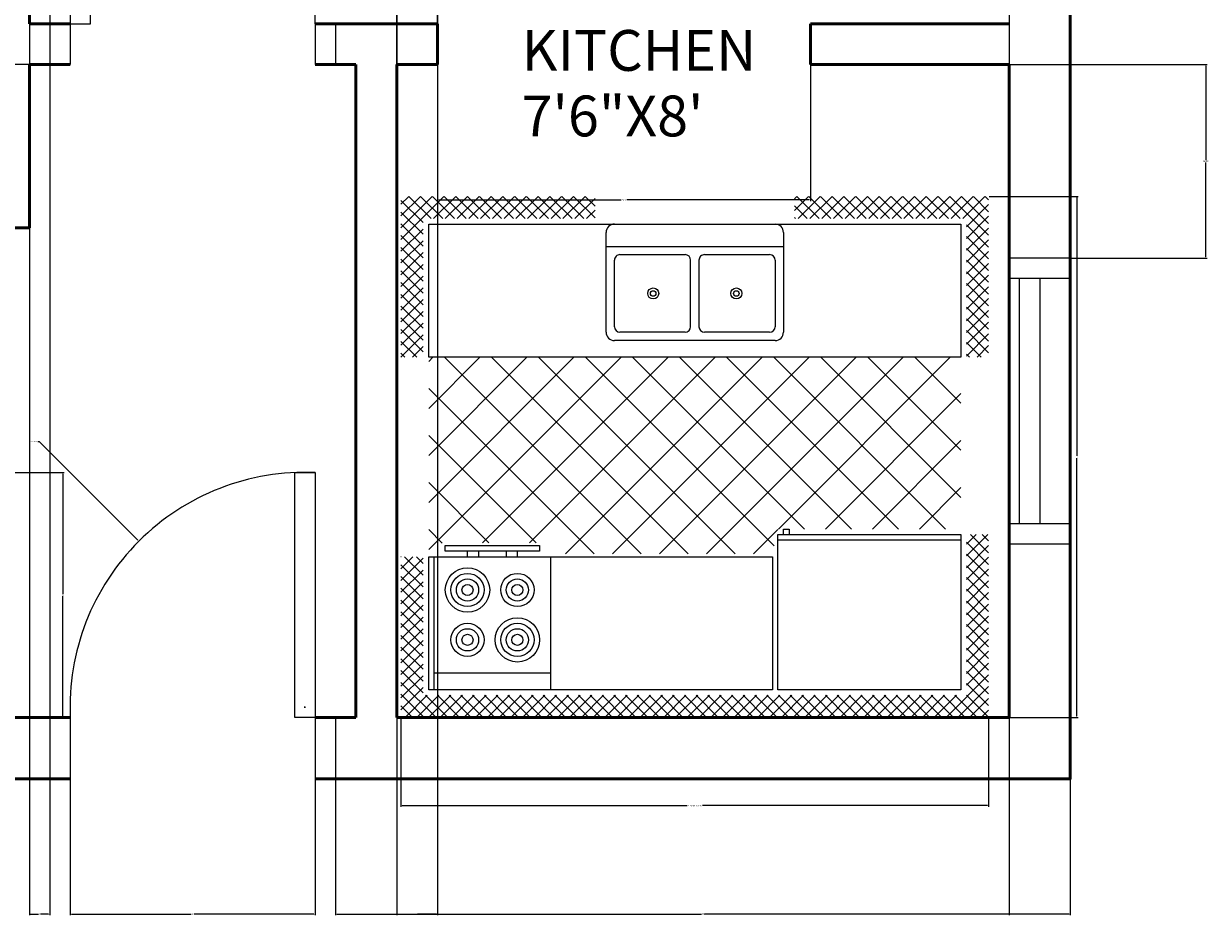
# Model space of a CAD drawing. Units: inches. Extents: x 2630 to 2982, y 643 to 1079.
# Tile 2 of 4: x 2808 to 2982, y 643 to 774. Entities that reach past the tile are written whole.
import ezdxf

# ---------------------------------------------------------------- set-up
doc = ezdxf.new("R2010")
doc.units = ezdxf.units.IN
for name, color, linetype, lineweight in [('A-ANNO-DIMS', 2, 'Continuous', 18), ('A-AREA-IDEN', 7, 'Continuous', 25), ('A-DOOR', 3, 'Continuous', 25), ('A-FLOR-FIXT', 9, 'Continuous', 18), ('A-GLAZ', 4, 'Continuous', 18), ('A-WALL', 7, 'Continuous', 50)]:
    doc.layers.add(name, color=color, linetype=linetype, lineweight=lineweight)
doc.styles.get("Standard").update_dxf_attribs({"font": 'arial.ttf'})
doc.dimstyles.get("Standard").update_dxf_attribs({"dimtxt": 0.18, "dimasz": 0.18, "dimexe": 0.18, "dimexo": 0.0625, "dimgap": 0.09, "dimtad": 0, "dimtih": 1, "dimtoh": 1, "dimdec": 4, "dimzin": 0, "dimdsep": 46, "dimtxsty": 'Standard', "dimcen": 0.09, "dimadec": 0, "dimazin": 0, "dimtfac": 1, "dimtdec": 4, "dimtofl": 0, "dimtmove": 0, "dimatfit": 3, "dimfxl": 1, "dimtolj": 1, "dimtzin": 0, "dimarcsym": 0})

# ---------------------------------------------------------------- blocks, each defined once
blk = doc.blocks.new('Kitchen Layout - 7 x 8 ft')
for p, q in [((-5, 81.32), (2.68, 89)), ((-5, 83.44), (0.56, 89)), ((-5, 85.56), (-1.56, 89)), ((-5, 87.68), (-3.68, 89)), ((-1, 84.97), (-5, 88.97)), ((1.09, 85), (-2.91, 89)), ((3.21, 85), (-0.79, 89)), ((0.81, 85), (4.81, 89)), ((5.34, 85), (1.34, 89)), ((2.93, 85), (6.93, 89)), ((7.46, 85), (3.46, 89)), ((5.05, 85), (9.05, 89)), ((9.58, 85), (5.58, 89)), ((7.17, 85), (11.17, 89)), ((11.7, 85), (7.7, 89)), ((9.29, 85), (13.29, 89)), ((13.82, 85), (9.82, 89)), ((11.41, 85), (15.41, 89)), ((15.94, 85), (11.94, 89)), ((13.53, 85), (17.53, 89)), ((18.06, 85), (14.06, 89)), ((15.65, 85), (19.65, 89)), ((20.18, 85), (16.18, 89)), ((17.78, 85), (21.78, 89)), ((22.31, 85), (18.31, 89)), ((19.9, 85), (23.9, 89)), ((24.43, 85), (20.43, 89)), ((22.02, 85), (26.02, 89)), ((26.55, 85), (22.55, 89)), ((24.14, 85), (28.14, 89)), ((28.67, 85), (24.67, 89)), ((26.26, 85), (30.26, 89)), ((30.79, 85), (26.79, 89)), ((28.38, 85), (32.38, 89)), ((32.91, 85), (28.91, 89)), ((30.5, 85), (34.5, 89)), ((35.03, 85), (31.03, 89)), ((32.63, 85), (36.63, 89)), ((37.16, 85), (33.16, 89)), ((34.75, 85), (38.75, 89)), ((39.28, 85), (35.28, 89)), ((36.87, 85), (40.87, 89)), ((41.4, 85), (37.4, 89)), ((38.99, 85), (42.99, 89)), ((43.52, 85), (39.52, 89)), ((41.11, 85), (45.11, 89)), ((45.64, 85), (41.64, 89)), ((43.23, 85), (47.23, 89)), ((47.76, 85), (43.76, 89)), ((45.35, 85), (49.35, 89)), ((49.88, 85), (45.88, 89)), ((47.47, 85), (51.47, 89)), ((52, 85), (48, 89)), ((49.6, 85), (53.6, 89)), ((54.13, 85), (50.13, 89)), ((51.72, 85), (55.72, 89)), ((56.25, 85), (52.25, 89)), ((53.84, 85), (57.84, 89)), ((58.37, 85), (54.37, 89)), ((55.96, 85), (59.96, 89)), ((60.49, 85), (56.49, 89)), ((58.08, 85), (62.08, 89)), ((62.61, 85), (58.61, 89)), ((60.2, 85), (64.2, 89)), ((64.73, 85), (60.73, 89)), ((62.32, 85), (66.32, 89)), ((66.85, 85), (62.85, 89)), ((64.45, 85), (68.45, 89)), ((68.97, 85), (64.97, 89)), ((66.57, 85), (70.57, 89)), ((71.1, 85), (67.1, 89)), ((68.69, 85), (72.69, 89)), ((73.22, 85), (69.22, 89)), ((70.81, 85), (74.81, 89)), ((75.34, 85), (71.34, 89)), ((72.93, 85), (76.93, 89)), ((77.46, 85), (73.46, 89)), ((75.05, 85), (79.05, 89)), ((79.58, 85), (75.58, 89)), ((77.17, 85), (81.17, 89)), ((81.7, 85), (77.7, 89)), ((79.29, 85), (83.29, 89)), ((83.82, 85), (79.82, 89)), ((81.42, 85), (85.42, 89)), ((85.95, 85), (81.95, 89)), ((83.54, 85), (87.54, 89)), ((88.07, 85), (84.07, 89)), ((85.66, 85), (89.66, 89)), ((90.19, 85), (86.19, 89)), ((87.78, 85), (91.78, 89)), ((92.31, 85), (88.31, 89)), ((89.9, 85), (93.9, 89)), ((94.43, 85), (90.43, 89)), ((92.02, 85), (96.02, 89)), ((96.55, 85), (92.55, 89)), ((94.14, 85), (98.14, 89)), ((101, 82.67), (94.67, 89)), ((96.27, 85), (100.27, 89)), ((101, 84.79), (96.79, 89)), ((97, 83.61), (101, 87.61)), ((101, 86.92), (98.92, 89)), ((-1, 82.85), (-5, 86.85)), ((97, 81.49), (101, 85.49)), ((-1, 80.73), (-5, 84.73)), ((34, 84), (96, 84)), ((34, 60), (34, 84)), ((96, 84), (96, 60)), ((101, 80.55), (97, 84.55)), ((97, 79.37), (101, 83.37)), ((-5, 79.19), (-1, 83.19)), ((-1, 78.61), (-5, 82.61)), ((101, 78.43), (97, 82.43)), ((97, 77.25), (101, 81.25)), ((-5, 77.07), (-1, 81.07)), ((-1, 76.49), (-5, 80.49)), ((74, 81), (95, 81)), ((101, 76.31), (97, 80.31)), ((97, 75.13), (101, 79.13)), ((-5, 74.95), (-1, 78.95)), ((-1, 74.36), (-5, 78.36)), ((101, 74.19), (97, 78.19)), ((97, 73.01), (101, 77.01)), ((-5, 72.83), (-1, 76.83)), ((-1, 72.24), (-5, 76.24)), ((101, 72.07), (97, 76.07)), ((97, 70.89), (101, 74.89)), ((-5, 70.71), (-1, 74.71)), ((-1, 70.12), (-5, 74.12)), ((101, 69.95), (97, 73.95)), ((97, 68.76), (101, 72.76)), ((-5, 68.59), (-1, 72.59)), ((-1, 68), (-5, 72)), ((101, 67.82), (97, 71.82)), ((97, 66.64), (101, 70.64)), ((-5, 66.47), (-1, 70.47)), ((-1, 65.88), (-5, 69.88)), ((101, 65.7), (97, 69.7)), ((97, 64.52), (101, 68.52)), ((-5, 64.35), (-1, 68.35)), ((-1, 63.76), (-5, 67.76)), ((101, 63.58), (97, 67.58)), ((97, 62.4), (101, 66.4)), ((-5, 62.22), (-1, 66.22)), ((-1, 61.64), (-5, 65.64)), ((101, 61.46), (97, 65.46)), ((97, 60.28), (101, 64.28)), ((-5, 60.1), (-1, 64.1)), ((-1, 59.52), (-5, 63.52)), ((-5, 57.98), (-1, 61.98)), ((100.34, 60), (97, 63.34)), ((98.84, 60), (101, 62.16)), ((-1, 57.39), (-5, 61.39)), ((-4.86, 56), (-1, 59.86)), ((96, 60), (34, 60)), ((80, 60), (80, 59)), ((82, 59), (82, 60)), ((87, 59), (87, 60)), ((89, 60), (89, 59)), ((98.22, 60), (97, 61.22)), ((100.96, 60), (101, 60.04)), ((-1.73, 56), (-5, 59.27)), ((-2.74, 56), (-1, 57.74)), ((10.4, 24), (45.9, 59.5)), ((18.88, 24), (54.38, 59.5)), ((27.37, 24), (62.87, 59.5)), ((33.03, 55.11), (37.41, 59.5)), ((67.71, 24), (33.68, 58.04)), ((35.85, 24), (71.35, 59.5)), ((76.2, 24), (40.7, 59.5)), ((84.68, 24), (49.18, 59.5)), ((93.17, 24), (57.67, 59.5)), ((61.31, 24), (96, 58.69)), ((96, 29.65), (66.15, 59.5)), ((-3.85, 56), (-5, 57.15)), ((0, 57), (33, 57)), ((31, 55), (31, 56)), ((32, 56), (32, 55)), ((44.34, 24), (77.84, 57.5)), ((52.82, 24), (86.32, 57.5)), ((96, 38.14), (76.64, 57.5)), ((96, 46.63), (85.13, 57.5)), ((96, 55.11), (93.57, 57.54)), ((0, 30.57), (24.43, 55)), ((0, 39.06), (15.94, 55)), ((0, 47.54), (7.46, 55)), ((1.91, 24), (32.91, 55)), ((33.77, 24), (2.77, 55)), ((42.26, 24), (11.26, 55)), ((50.74, 24), (19.74, 55)), ((59.23, 24), (28.23, 55)), ((32, 55), (31, 55)), ((25.29, 24), (0, 49.29)), ((69.79, 24), (96, 50.21)), ((16.8, 24), (0, 40.8)), ((78.28, 24), (96, 41.72)), ((8.32, 24), (0, 32.32)), ((86.76, 24), (96, 33.24)), ((-5, 21.92), (-2.92, 24)), ((-5, 19.8), (-1, 23.8)), ((-1, 21.33), (-3.67, 24)), ((-1, 23.45), (-1.55, 24)), ((0, 24), (96, 24)), ((0, 0), (0, 24)), ((95.25, 24), (96, 24.75)), ((96, 24), (96, 0)), ((97, 22.1), (98.9, 24)), ((97, 19.97), (101, 23.97)), ((101, 21.16), (98.16, 24)), ((101, 23.28), (100.28, 24)), ((-1, 19.21), (-5, 23.21)), ((-5, 17.68), (-1, 21.68)), ((101, 19.03), (97, 23.03)), ((97, 17.85), (101, 21.85)), ((-1, 17.09), (-5, 21.09)), ((-5, 15.55), (-1, 19.55)), ((101, 16.91), (97, 20.91)), ((97, 15.73), (101, 19.73)), ((-1, 14.97), (-5, 18.97)), ((-5, 13.43), (-1, 17.43)), ((47.25, 6.5), (47.25, 18.5)), ((48.75, 18.5), (48.75, 6.5)), ((101, 14.79), (97, 18.79)), ((97, 13.61), (101, 17.61)), ((-1, 12.85), (-5, 16.85)), ((-5, 11.31), (-1, 15.31)), ((101, 12.67), (97, 16.67)), ((97, 11.49), (101, 15.49)), ((-1, 10.73), (-5, 14.73)), ((-5, 9.19), (-1, 13.19)), ((101, 10.55), (97, 14.55)), ((97, 9.37), (101, 13.37)), ((-1, 8.6), (-5, 12.6)), ((-5, 7.07), (-1, 11.07)), ((101, 8.43), (97, 12.43)), ((97, 7.25), (101, 11.25)), ((-1, 6.48), (-5, 10.48)), ((-5, 4.95), (-1, 8.95)), ((101, 6.31), (97, 10.31)), ((97, 5.12), (101, 9.12)), ((-1, 4.36), (-5, 8.36)), ((-5, 2.83), (-1, 6.83)), ((101, 4.18), (97, 8.18)), ((97, 3), (101, 7)), ((-1, 2.24), (-5, 6.24)), ((-5, 0.71), (-1, 4.71)), ((101, 2.06), (97, 6.06)), ((97, 0.88), (101, 4.88)), ((-1, 0.12), (-5, 4.12)), ((-5, -1.42), (-1, 2.58)), ((64, 4), (32, 4)), ((93.24, -5), (101, 2.76)), ((101, -0.06), (97, 3.94)), ((2, -5), (-5, 2)), ((-5, -3.54), (-1, 0.46)), ((96, 0), (0, 0)), ((95.36, -5), (101, 0.64)), ((101, -2.18), (97, 1.82)), ((-0.12, -5), (-5, -0.12)), ((-4.34, -5), (-0.34, -1)), ((-2.22, -5), (1.78, -1)), ((-0.1, -5), (3.9, -1)), ((4.12, -5), (0.12, -1)), ((2.02, -5), (6.02, -1)), ((6.24, -5), (2.24, -1)), ((4.14, -5), (8.14, -1)), ((8.36, -5), (4.36, -1)), ((6.27, -5), (10.27, -1)), ((10.48, -5), (6.48, -1)), ((8.39, -5), (12.39, -1)), ((12.6, -5), (8.6, -1)), ((10.51, -5), (14.51, -1)), ((14.73, -5), (10.73, -1)), ((12.63, -5), (16.63, -1)), ((16.85, -5), (12.85, -1)), ((14.75, -5), (18.75, -1)), ((18.97, -5), (14.97, -1)), ((16.87, -5), (20.87, -1)), ((21.09, -5), (17.09, -1)), ((18.99, -5), (22.99, -1)), ((23.21, -5), (19.21, -1)), ((21.11, -5), (25.11, -1)), ((25.33, -5), (21.33, -1)), ((23.24, -5), (27.24, -1)), ((27.45, -5), (23.45, -1)), ((25.36, -5), (29.36, -1)), ((29.57, -5), (25.57, -1)), ((30, -3.3), (27.7, -1)), ((30, -1.18), (29.82, -1)), ((66, -2.54), (67.54, -1)), ((66, -4.66), (69.66, -1)), ((69.88, -5), (66, -1.12)), ((67.78, -5), (71.78, -1)), ((72, -5), (68, -1)), ((69.9, -5), (73.9, -1)), ((74.12, -5), (70.12, -1)), ((72.03, -5), (76.03, -1)), ((76.24, -5), (72.24, -1)), ((74.15, -5), (78.15, -1)), ((78.36, -5), (74.36, -1)), ((76.27, -5), (80.27, -1)), ((80.49, -5), (76.49, -1)), ((78.39, -5), (82.39, -1)), ((82.61, -5), (78.61, -1)), ((80.51, -5), (84.51, -1)), ((84.73, -5), (80.73, -1)), ((82.63, -5), (86.63, -1)), ((86.85, -5), (82.85, -1)), ((84.75, -5), (88.75, -1)), ((88.97, -5), (84.97, -1)), ((86.88, -5), (90.88, -1)), ((91.09, -5), (87.09, -1)), ((89, -5), (93, -1)), ((93.21, -5), (89.21, -1)), ((91.12, -5), (95.12, -1)), ((95.34, -5), (91.34, -1)), ((97.46, -5), (93.46, -1)), ((99.58, -5), (95.58, -1)), ((101, -4.3), (97, -0.3)), ((97.48, -5), (101, -1.48)), ((-2.25, -5), (-5, -2.25)), ((27.48, -5), (30, -2.48)), ((67.76, -5), (66, -3.24)), ((99.6, -5), (101, -3.6)), ((-4.37, -5), (-5, -4.37)), ((29.6, -5), (30, -4.6))]:
    blk.add_line(p, q)
for points in [[(0, 56), (0, 84), (33, 84), (33, 56)], [(74, 60), (74, 84), (95, 84), (95, 60)], [(76, 58), (76, 59), (93, 59), (93, 58)]]:
    blk.add_lwpolyline(points, close=True)
for points in [[(32, 1.5), (32, 19.5)], [(33.5, 21), (62.5, 21)], [(34.5, 19.5), (46.25, 19.5)], [(49.75, 19.5), (61.5, 19.5)], [(64, 19.5), (64, 1.5)], [(33.5, 6.5), (33.5, 18.5)], [(62.5, 18.5), (62.5, 6.5)], [(46.25, 5.5), (34.5, 5.5)], [(61.5, 5.5), (49.75, 5.5)], [(62.5, 0), (33.5, 0)]]:
    blk.add_lwpolyline(points)
for centre, radius in [((80, 75), 4), ((80, 75), 3), ((80, 75), 2), ((89, 75), 3), ((89, 75), 2), ((80, 75), 1), ((89, 75), 1), ((80, 66), 3), ((89, 66), 4), ((89, 66), 3), ((80, 66), 2), ((80, 66), 1), ((89, 66), 2), ((89, 66), 1), ((40.5, 12.5), 1), ((40.5, 12.5), 0.5), ((55.5, 12.5), 1), ((55.5, 12.5), 0.5)]:
    blk.add_circle(centre, radius)
for centre, radius, start, end in [((33.5, 19.5), 1.5, 90, 180), ((34.5, 18.5), 1, 90, 180), ((46.25, 18.5), 1, 0, 90), ((49.75, 18.5), 1, 90, 180), ((61.5, 18.5), 1, 0, 90), ((62.5, 19.5), 1.5, 0, 90), ((34.5, 6.5), 1, 180, 270), ((46.25, 6.5), 1, 270, 0), ((49.75, 6.5), 1, 180, 270), ((61.5, 6.5), 1, 270, 0), ((33.5, 1.5), 1.5, 180, 270), ((62.5, 1.5), 1.5, 270, 0)]:
    blk.add_arc(centre, radius, start, end)
blk = doc.blocks.new('DOOR-36IN-INT')
for p, q in [((0, 6), (0, 0)), ((3, 6), (3, 0)), ((39, 6), (39, 0)), ((42, 6), (42, 0))]:
    blk.add_line(p, q)
blk.add_lwpolyline([(3, 6), (6, 6), (6, 42), (3, 42)], close=True)
blk.add_arc((4.5, 7.5), 34.53, 357.5104, 92.4896)
blk = doc.blocks.new('WIN-36IN')
for p, q in [((9, 42), (0, 42)), ((9, 39), (0, 39)), ((4.5, 3), (4.5, 39)), ((7.5, 3), (7.5, 39)), ((0, 3), (9, 3)), ((0, 0), (9, 0))]:
    blk.add_line(p, q)
blk = doc.blocks.new('*D19')
at = {"layer": 'A-ANNO-DIMS', "color": 0, "lineweight": -2, "transparency": 16777216}
for p, q in [((2811.7, 810.29), (2805.22, 810.29)), ((2805.4, 810.11), (2805.4, 789.26)), ((2805.4, 768.05), (2805.4, 788.89)), ((2811.7, 767.87), (2805.22, 767.87))]:
    blk.add_line(p, q, dxfattribs=at)
at = {"layer": 'A-ANNO-DIMS', "color": 0, "transparency": 16777216}
for points in [[(2805.37, 810.11), (2805.43, 810.11), (2805.4, 810.29)], [(2805.37, 768.05), (2805.43, 768.05), (2805.4, 767.87)]]:
    blk.add_solid(points, dxfattribs=at)
at = {"layer": 'Defpoints', "color": 0, "transparency": 16777216}
for p in [(2805.4, 810.29), (2811.77, 810.29), (2811.77, 767.87)]:
    blk.add_point(p, dxfattribs=at)
at = {"layer": 'A-ANNO-DIMS', "color": 0, "transparency": 16777216, "insert": (2805.4, 789.08), "char_height": 0.18, "attachment_point": 5}
blk.add_mtext('\\A1;DOOR D1 42 TYP.', dxfattribs=at)
blk = doc.blocks.new('*D35')
at = {"layer": 'A-ANNO-DIMS', "color": 0, "lineweight": -2, "transparency": 16777216}
for p, q in [((2863.38, 671.8), (2863.38, 658.73)), ((2949.76, 671.8), (2949.76, 658.73)), ((2863.56, 658.91), (2905.44, 658.91)), ((2949.58, 658.91), (2907.7, 658.91))]:
    blk.add_line(p, q, dxfattribs=at)
at = {"layer": 'A-ANNO-DIMS', "color": 0, "transparency": 16777216}
for points in [[(2863.56, 658.94), (2863.56, 658.88), (2863.38, 658.91)], [(2949.58, 658.94), (2949.58, 658.88), (2949.76, 658.91)]]:
    blk.add_solid(points, dxfattribs=at)
at = {"layer": 'Defpoints', "color": 0, "transparency": 16777216}
for p in [(2863.38, 671.87), (2949.76, 671.87), (2863.38, 658.91)]:
    blk.add_point(p, dxfattribs=at)
at = {"layer": 'A-ANNO-DIMS', "color": 0, "transparency": 16777216, "insert": (2906.57, 658.91), "char_height": 0.18, "attachment_point": 5}
blk.add_mtext('\\A1;KITCHEN UNIT 86', dxfattribs=at)
blk = doc.blocks.new('*D36')
at = {"layer": 'A-ANNO-DIMS', "color": 0, "lineweight": -2, "transparency": 16777216}
for p, q in [((2949.82, 748.47), (2962.9, 748.47)), ((2962.72, 748.29), (2962.72, 710.35)), ((2962.72, 672.05), (2962.72, 709.99)), ((2949.82, 671.87), (2962.9, 671.87))]:
    blk.add_line(p, q, dxfattribs=at)
at = {"layer": 'A-ANNO-DIMS', "color": 0, "transparency": 16777216}
for points in [[(2962.69, 748.29), (2962.75, 748.29), (2962.72, 748.47)], [(2962.69, 672.05), (2962.75, 672.05), (2962.72, 671.87)]]:
    blk.add_solid(points, dxfattribs=at)
at = {"layer": 'Defpoints', "color": 0, "transparency": 16777216}
for p in [(2949.76, 748.47), (2949.76, 671.87), (2962.72, 671.87)]:
    blk.add_point(p, dxfattribs=at)
at = {"layer": 'A-ANNO-DIMS', "color": 0, "transparency": 16777216, "insert": (2962.72, 710.17), "char_height": 0.18, "attachment_point": 5}
blk.add_mtext('\\A1;77', dxfattribs=at)
blk = doc.blocks.new('*D48')
at = {"layer": 'A-ANNO-DIMS', "color": 0, "lineweight": -2, "transparency": 16777216}
for p, q in [((2952.83, 767.87), (2981.86, 767.87)), ((2981.68, 767.69), (2981.68, 753.81)), ((2981.68, 739.57), (2981.68, 753.45)), ((2961.83, 739.39), (2981.86, 739.39))]:
    blk.add_line(p, q, dxfattribs=at)
at = {"layer": 'A-ANNO-DIMS', "color": 0, "transparency": 16777216}
for points in [[(2981.65, 767.69), (2981.71, 767.69), (2981.68, 767.87)], [(2981.65, 739.57), (2981.71, 739.57), (2981.68, 739.39)]]:
    blk.add_solid(points, dxfattribs=at)
at = {"layer": 'Defpoints', "color": 0, "transparency": 16777216}
for p in [(2952.77, 767.87), (2981.68, 767.87), (2961.77, 739.39)]:
    blk.add_point(p, dxfattribs=at)
at = {"layer": 'A-ANNO-DIMS', "color": 0, "transparency": 16777216, "insert": (2981.68, 753.63), "char_height": 0.18, "attachment_point": 5}
blk.add_mtext('\\A1;28.475', dxfattribs=at)
blk = doc.blocks.new('*D49')
at = {"layer": 'A-ANNO-DIMS', "color": 0, "lineweight": -2, "transparency": 16777216}
for p, q in [((2853.77, 662.8), (2853.77, 642.78)), ((2961.77, 662.8), (2961.77, 642.78)), ((2853.95, 642.96), (2907.49, 642.96)), ((2961.59, 642.96), (2908.05, 642.96))]:
    blk.add_line(p, q, dxfattribs=at)
at = {"layer": 'A-ANNO-DIMS', "color": 0, "transparency": 16777216}
for points in [[(2853.95, 642.99), (2853.95, 642.93), (2853.77, 642.96)], [(2961.59, 642.99), (2961.59, 642.93), (2961.77, 642.96)]]:
    blk.add_solid(points, dxfattribs=at)
at = {"layer": 'Defpoints', "color": 0, "transparency": 16777216}
for p in [(2853.77, 662.87), (2961.77, 662.87), (2961.77, 642.96)]:
    blk.add_point(p, dxfattribs=at)
at = {"layer": 'A-ANNO-DIMS', "color": 0, "transparency": 16777216, "insert": (2907.77, 642.96), "char_height": 0.18, "attachment_point": 5}
blk.add_mtext('\\A1;108', dxfattribs=at)
blk = doc.blocks.new('*D50')
at = {"layer": 'A-ANNO-DIMS', "color": 0, "lineweight": -2, "transparency": 16777216}
for p, q in [((2814.77, 662.8), (2814.77, 642.78)), ((2850.77, 662.8), (2850.77, 642.78)), ((2814.95, 642.96), (2832.55, 642.96)), ((2850.59, 642.96), (2832.99, 642.96))]:
    blk.add_line(p, q, dxfattribs=at)
at = {"layer": 'A-ANNO-DIMS', "color": 0, "transparency": 16777216}
for points in [[(2814.95, 642.99), (2814.95, 642.93), (2814.77, 642.96)], [(2850.59, 642.99), (2850.59, 642.93), (2850.77, 642.96)]]:
    blk.add_solid(points, dxfattribs=at)
at = {"layer": 'Defpoints', "color": 0, "transparency": 16777216}
for p in [(2814.77, 662.87), (2850.77, 662.87), (2850.77, 642.96)]:
    blk.add_point(p, dxfattribs=at)
at = {"layer": 'A-ANNO-DIMS', "color": 0, "transparency": 16777216, "insert": (2832.77, 642.96), "char_height": 0.18, "attachment_point": 5}
blk.add_mtext('\\A1;36', dxfattribs=at)
blk = doc.blocks.new('*D51')
at = {"layer": 'A-ANNO-DIMS', "color": 0, "lineweight": -2, "transparency": 16777216}
for p, q in [((2862.77, 875.8), (2862.77, 642.78)), ((2952.77, 875.8), (2952.77, 642.78)), ((2862.95, 642.96), (2907.55, 642.96)), ((2952.59, 642.96), (2907.99, 642.96))]:
    blk.add_line(p, q, dxfattribs=at)
at = {"layer": 'A-ANNO-DIMS', "color": 0, "transparency": 16777216}
for points in [[(2862.95, 642.99), (2862.95, 642.93), (2862.77, 642.96)], [(2952.59, 642.99), (2952.59, 642.93), (2952.77, 642.96)]]:
    blk.add_solid(points, dxfattribs=at)
at = {"layer": 'Defpoints', "color": 0, "transparency": 16777216}
for p in [(2862.77, 875.87), (2952.77, 875.87), (2952.77, 642.96)]:
    blk.add_point(p, dxfattribs=at)
at = {"layer": 'A-ANNO-DIMS', "color": 0, "transparency": 16777216, "insert": (2907.77, 642.96), "char_height": 0.18, "attachment_point": 5}
blk.add_mtext('\\A1;90', dxfattribs=at)
blk = doc.blocks.new('*D53')
at = {"layer": 'A-ANNO-DIMS', "color": 0, "lineweight": -2, "transparency": 16777216}
for p, q in [((2793.83, 707.87), (2813.86, 707.87)), ((2813.68, 707.69), (2813.68, 690.05)), ((2813.68, 672.05), (2813.68, 689.68)), ((2793.83, 671.87), (2813.86, 671.87))]:
    blk.add_line(p, q, dxfattribs=at)
at = {"layer": 'A-ANNO-DIMS', "color": 0, "transparency": 16777216}
for points in [[(2813.65, 707.69), (2813.71, 707.69), (2813.68, 707.87)], [(2813.65, 672.05), (2813.71, 672.05), (2813.68, 671.87)]]:
    blk.add_solid(points, dxfattribs=at)
at = {"layer": 'Defpoints', "color": 0, "transparency": 16777216}
for p in [(2793.77, 707.87), (2793.77, 671.87), (2813.68, 671.87)]:
    blk.add_point(p, dxfattribs=at)
at = {"layer": 'A-ANNO-DIMS', "color": 0, "transparency": 16777216, "insert": (2813.68, 689.87), "char_height": 0.18, "attachment_point": 5}
blk.add_mtext('\\A1;36', dxfattribs=at)
blk = doc.blocks.new('*D57')
at = {"layer": 'A-ANNO-DIMS', "color": 0, "lineweight": -2, "transparency": 16777216}
for p, q in [((2868.77, 767.8), (2868.77, 747.78)), ((2923.56, 767.8), (2923.56, 747.78)), ((2868.95, 747.96), (2895.77, 747.96)), ((2923.38, 747.96), (2896.56, 747.96))]:
    blk.add_line(p, q, dxfattribs=at)
at = {"layer": 'A-ANNO-DIMS', "color": 0, "transparency": 16777216}
for points in [[(2868.95, 747.99), (2868.95, 747.93), (2868.77, 747.96)], [(2923.38, 747.99), (2923.38, 747.93), (2923.56, 747.96)]]:
    blk.add_solid(points, dxfattribs=at)
at = {"layer": 'Defpoints', "color": 0, "transparency": 16777216}
for p in [(2868.77, 767.87), (2923.56, 767.87), (2868.77, 747.96)]:
    blk.add_point(p, dxfattribs=at)
at = {"layer": 'A-ANNO-DIMS', "color": 0, "transparency": 16777216, "insert": (2896.16, 747.96), "char_height": 0.18, "attachment_point": 5}
blk.add_mtext('\\A1;54.79', dxfattribs=at)
blk = doc.blocks.new('*D58')
at = {"layer": 'A-ANNO-DIMS', "color": 0, "lineweight": -2, "transparency": 16777216}
for p, q in [((2862.77, 767.93), (2862.77, 1078.96)), ((2862.95, 1078.78), (2865.62, 1078.78)), ((2868.59, 1078.78), (2865.92, 1078.78)), ((2868.77, 767.93), (2868.77, 1078.96))]:
    blk.add_line(p, q, dxfattribs=at)
at = {"layer": 'A-ANNO-DIMS', "color": 0, "transparency": 16777216}
for points in [[(2862.95, 1078.81), (2862.95, 1078.75), (2862.77, 1078.78)], [(2868.59, 1078.81), (2868.59, 1078.75), (2868.77, 1078.78)]]:
    blk.add_solid(points, dxfattribs=at)
at = {"layer": 'Defpoints', "color": 0, "transparency": 16777216}
for p in [(2868.77, 1078.78), (2862.77, 767.87), (2868.77, 767.87)]:
    blk.add_point(p, dxfattribs=at)
at = {"layer": 'A-ANNO-DIMS', "color": 0, "transparency": 16777216, "insert": (2865.77, 1078.78), "char_height": 0.18, "attachment_point": 5}
blk.add_mtext('\\A1;6', dxfattribs=at)
blk = doc.blocks.new('*D59')
at = {"layer": 'A-ANNO-DIMS', "color": 0, "lineweight": -2, "transparency": 16777216}
for p, q in [((2808.77, 929.8), (2808.77, 642.78)), ((2811.77, 929.8), (2811.77, 642.78)), ((2808.95, 642.96), (2810.12, 642.96)), ((2811.59, 642.96), (2810.42, 642.96))]:
    blk.add_line(p, q, dxfattribs=at)
at = {"layer": 'A-ANNO-DIMS', "color": 0, "transparency": 16777216}
for points in [[(2808.95, 642.99), (2808.95, 642.93), (2808.77, 642.96)], [(2811.59, 642.99), (2811.59, 642.93), (2811.77, 642.96)]]:
    blk.add_solid(points, dxfattribs=at)
at = {"layer": 'Defpoints', "color": 0, "transparency": 16777216}
for p in [(2808.77, 929.87), (2811.77, 929.87), (2811.77, 642.96)]:
    blk.add_point(p, dxfattribs=at)
at = {"layer": 'A-ANNO-DIMS', "color": 0, "transparency": 16777216, "insert": (2810.27, 642.96), "char_height": 0.18, "attachment_point": 5}
blk.add_mtext('\\A1;3', dxfattribs=at)
blk = doc.blocks.new('*D60')
at = {"layer": 'A-ANNO-DIMS', "color": 0, "lineweight": -2, "transparency": 16777216}
for p, q in [((2862.77, 923.8), (2862.77, 642.78)), ((2868.77, 923.8), (2868.77, 642.78)), ((2862.95, 642.96), (2865.62, 642.96)), ((2868.59, 642.96), (2865.92, 642.96))]:
    blk.add_line(p, q, dxfattribs=at)
at = {"layer": 'A-ANNO-DIMS', "color": 0, "transparency": 16777216}
for points in [[(2862.95, 642.99), (2862.95, 642.93), (2862.77, 642.96)], [(2868.59, 642.99), (2868.59, 642.93), (2868.77, 642.96)]]:
    blk.add_solid(points, dxfattribs=at)
at = {"layer": 'Defpoints', "color": 0, "transparency": 16777216}
for p in [(2862.77, 923.87), (2868.77, 923.87), (2868.77, 642.96)]:
    blk.add_point(p, dxfattribs=at)
at = {"layer": 'A-ANNO-DIMS', "color": 0, "transparency": 16777216, "insert": (2865.77, 642.96), "char_height": 0.18, "attachment_point": 5}
blk.add_mtext('\\A1;6', dxfattribs=at)
blk = doc.blocks.new('*D69')
at = {"layer": 'A-ANNO-DIMS', "color": 0, "lineweight": -2, "transparency": 16777216}
for p, q in [((2810.02, 712.44), (2810.2, 712.44)), ((2810.2, 712.44), (2824.72, 697.91)), ((2849.18, 673.37), (2849.36, 673.37)), ((2849.27, 673.28), (2849.27, 673.46))]:
    blk.add_line(p, q, dxfattribs=at)
at = {"layer": 'A-ANNO-DIMS', "color": 0, "transparency": 16777216}
blk.add_solid([(2824.74, 697.93), (2824.7, 697.89), (2824.85, 697.78)], dxfattribs=at)
at = {"layer": 'Defpoints', "color": 0, "transparency": 16777216}
for p in [(2824.85, 697.78), (2849.27, 673.37)]:
    blk.add_point(p, dxfattribs=at)
at = {"layer": 'A-ANNO-DIMS', "color": 0, "transparency": 16777216, "insert": (2809.34, 712.44), "char_height": 0.18, "attachment_point": 5}
blk.add_mtext('\\A1;4X R34.53', dxfattribs=at)

msp = doc.modelspace()

# ---------------------------------------------------------------- linework, layer by layer
at = {"layer": 'A-DOOR'}
for p, q in [((2811.7671, 671.8666), (2811.7671, 662.8666)), ((2814.7671, 671.8666), (2814.7671, 662.8666)), ((2850.7671, 671.8666), (2850.7671, 662.8666)), ((2853.7671, 671.8666), (2853.7671, 662.8666))]:
    msp.add_line(p, q, dxfattribs=at)
msp.add_lwpolyline([(2850.7671, 671.8666), (2847.7671, 671.8666), (2847.7671, 707.8666), (2850.7671, 707.8666)], close=True, dxfattribs=at)
msp.add_arc((2849.2671, 673.3666), 34.5326, 87.510447, 182.489553, dxfattribs=at)
at = {"layer": 'A-WALL'}
for p, q in [((2808.7671, 875.8666), (2808.7671, 773.8666)), ((2808.7671, 773.8666), (2814.7671, 773.8666)), ((2850.7671, 773.8666), (2868.7671, 773.8666)), ((2868.7671, 767.8666), (2868.7671, 773.8666)), ((2923.557, 773.8666), (2952.7671, 773.8666)), ((2923.557, 773.8666), (2923.557, 767.8666)), ((2808.7671, 767.8666), (2814.7671, 767.8666)), ((2808.7671, 767.8666), (2808.7671, 743.8666)), ((2850.7671, 767.8666), (2856.7671, 767.8666)), ((2856.7671, 671.8666), (2856.7671, 767.8666)), ((2862.7671, 671.8666), (2862.7671, 767.8666)), ((2862.7671, 767.8666), (2868.7671, 767.8666)), ((2923.557, 767.8666), (2952.7671, 767.8666)), ((2952.7671, 671.8666), (2952.7671, 767.8666)), ((2808.7671, 743.8666), (2658.7671, 743.8666)), ((2658.7671, 671.8666), (2814.7671, 671.8666)), ((2850.7671, 671.8666), (2856.7671, 671.8666)), ((2862.7671, 671.8666), (2952.7671, 671.8666))]:
    msp.add_line(p, q, dxfattribs=at)
msp.add_lwpolyline([(2850.7671, 662.8666), (2961.7671, 662.8666), (2961.7671, 1058.8666), (2649.7671, 1058.8666), (2649.7671, 662.8666), (2814.7671, 662.8666)], dxfattribs=at)

# ---------------------------------------------------------------- block references
at = {"layer": 'A-DOOR'}
msp.add_blockref('DOOR-36IN-INT', (2811.767, 767.867), dxfattribs=at)
at = {"layer": 'A-FLOR-FIXT', "xscale": 0.8148768357365197, "yscale": 0.8148768357365197, "zscale": 0.8148768357365197, "rotation": 180}
msp.add_blockref('Kitchen Layout - 7 x 8 ft', (2945.6847, 744.3907), dxfattribs=at)
at = {"layer": 'A-GLAZ', "rotation": 180}
msp.add_blockref('WIN-36IN', (2961.7672, 739.3914), dxfattribs=at)

# ---------------------------------------------------------------- texts
at = {"layer": 'A-AREA-IDEN'}
for s, p in [('KITCHEN', (2881.1094, 766.9372)), ('7\'6"X8\'', (2881.1094, 757.2987))]:
    msp.add_text(s, height=6, dxfattribs=at).set_placement(p)

# ---------------------------------------------------------------- dimensions: what is measured, and where the dimension line sits
at = {"layer": 'A-ANNO-DIMS'}
for base, p1, p2, picture, middle in [((2868.7671, 1078.7766), (2862.7671, 767.8666), (2868.7671, 767.8666), '*D58', (2865.7671, 1078.7766)), ((2811.7671, 642.9566), (2808.7671, 929.8666), (2811.7671, 929.8666), '*D59', (2810.2671, 642.9566)), ((2868.7671, 642.9566), (2862.7671, 923.8666), (2868.7671, 923.8666), '*D60', (2865.7671, 642.9566)), ((2952.7671, 642.9566), (2862.7671, 875.8666), (2952.7671, 875.8666), '*D51', (2907.7671, 642.9566)), ((2850.7671, 642.9566), (2814.7671, 662.8666), (2850.7671, 662.8666), '*D50', (2832.7671, 642.9566)), ((2961.7671, 642.9566), (2853.7671, 662.8666), (2961.7671, 662.8666), '*D49', (2907.7671, 642.9566))]:
    dim = msp.add_linear_dim(base=base, p1=p1, p2=p2, dimstyle='Standard', override={"dimdec": 0, "dimlfac": 1, "dimrnd": 0, "dimzin": 0, "dimdsep": 46, "dimlunit": 2}, dxfattribs=at)
    dim.commit()
    dim.dimension.update_dxf_attribs({"geometry": picture, "text_midpoint": middle})
for base, p1, p2, angle, text, picture, middle in [((2805.404, 810.2871), (2811.7671, 767.8666), (2811.7671, 810.2871), 90, 'DOOR D1 <> TYP.', '*D19', (2805.404, 789.0769)), ((2863.3821, 658.9101), (2949.7591, 671.8666), (2863.3821, 671.8666), 180, 'KITCHEN UNIT <>', '*D35', (2906.5706, 658.9101))]:
    dim = msp.add_linear_dim(base=base, p1=p1, p2=p2, angle=angle, text=text, dimstyle='Standard', override={"dimdec": 0, "dimlfac": 1, "dimrnd": 0, "dimzin": 0, "dimdsep": 46, "dimlunit": 2}, dxfattribs=at)
    dim.commit()
    dim.dimension.update_dxf_attribs({"geometry": picture, "text_midpoint": middle})
for base, p1, p2, angle, override, picture, middle in [((2868.7671, 747.9566), (2923.557, 767.8666), (2868.7671, 767.8666), 180, {"dimdec": 2, "dimlfac": 1, "dimrnd": 0, "dimzin": 0, "dimdsep": 46, "dimlunit": 2}, '*D57', (2896.162, 747.9566)), ((2981.6771, 767.8666), (2961.7671, 739.3915), (2952.7671, 767.8666), 90, {"dimdec": 3, "dimlfac": 1, "dimrnd": 0, "dimzin": 0, "dimdsep": 46, "dimlunit": 2}, '*D48', (2981.6771, 753.6291)), ((2962.7156, 671.8666), (2949.7591, 748.4651), (2949.7591, 671.8666), 270, {"dimdec": 0, "dimlfac": 1, "dimrnd": 0, "dimzin": 0, "dimdsep": 46, "dimlunit": 2}, '*D36', (2962.7156, 710.1658)), ((2813.6771, 671.8666), (2793.7671, 707.8666), (2793.7671, 671.8666), 270, {"dimdec": 0, "dimlfac": 1, "dimrnd": 0, "dimzin": 0, "dimdsep": 46, "dimlunit": 2}, '*D53', (2813.6771, 689.8666))]:
    dim = msp.add_linear_dim(base=base, p1=p1, p2=p2, angle=angle, dimstyle='Standard', override=override, dxfattribs=at)
    dim.commit()
    dim.dimension.update_dxf_attribs({"geometry": picture, "text_midpoint": middle})
dim = msp.add_radius_dim(center=(2849.2671, 673.3666), mpoint=(2824.849, 697.785), text='4X <>', dimstyle='Standard', override={"dimdec": 2, "dimlfac": 1, "dimrnd": 0, "dimzin": 0, "dimdsep": 46, "dimlunit": 2}, dxfattribs=at)
dim.commit()
dim.dimension.update_dxf_attribs({"geometry": '*D69', "text_midpoint": (2809.3413, 712.436), "dimtype": 164})

doc.saveas('drawing.dxf')
